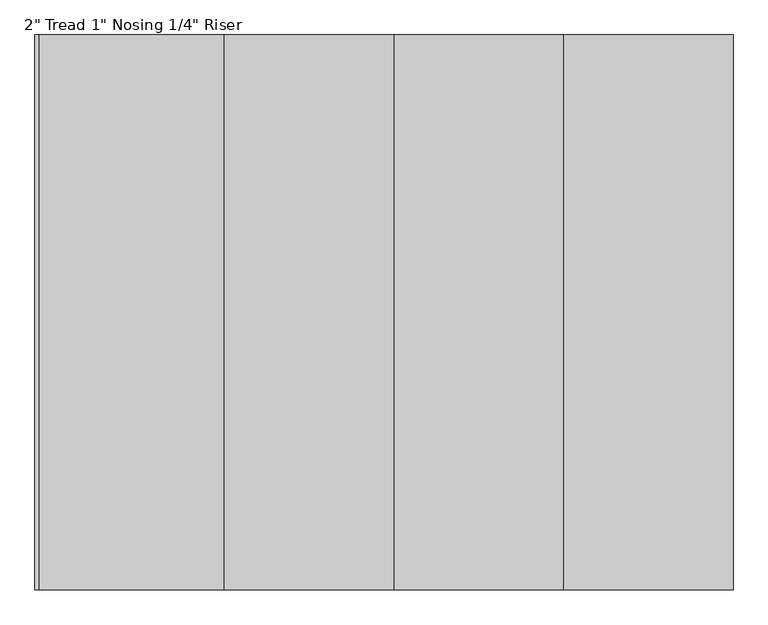
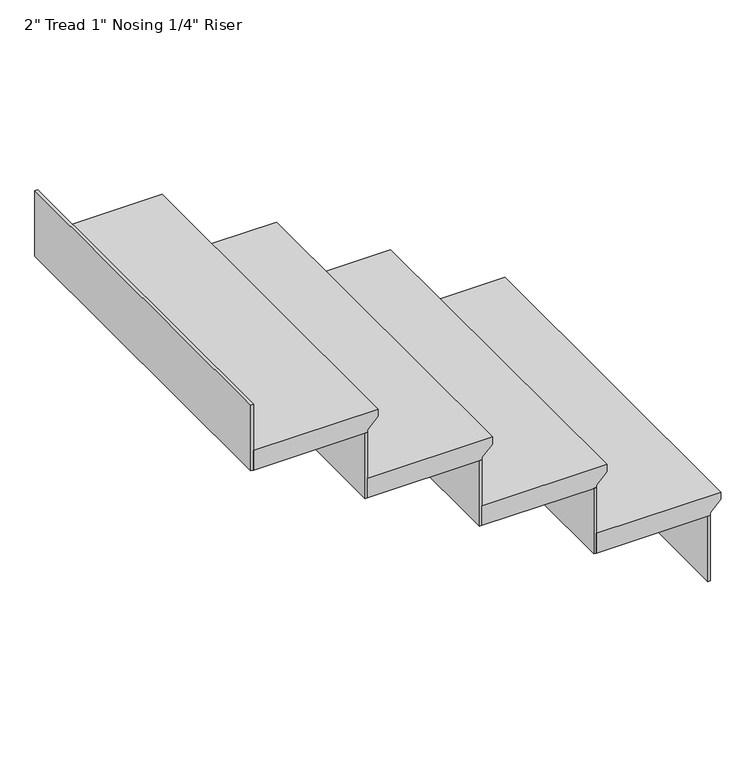
"""IFC4 building model written with IfcOpenShell, lengths in millimetres: stair flight geometry."""

from ifc_helpers import new_model, si_unit, frame, origin, place, context, project, spatial, polyline, outline, extrude, source, transform, mapped, element, save


def stair_flight_6800fc22(model_context):
    return source(origin(), model_context, "Body", "SweptSolid", [
        extrude(outline(polyline([(1016.0, -7602.2399968), (1016.0, -7907.0399968), (965.2, -7907.0399968), (965.2, -7627.6399968), (971.55, -7627.6399968), (996.95, -7602.2399968), (1016.0, -7602.2399968)])), frame((0.0, 8083.4426639, 0.0), z_axis=(0.0, 1.0, 0.0), x_axis=(0.0, 0.0, 1.0)), (0.0, 0.0, 1.0), 914.4),
        extrude(outline(polyline([(-7633.9899968, 8997.8426639), (-7627.6399968, 8997.8426639), (-7627.6399968, 8083.4426639), (-7633.9899968, 8083.4426639), (-7633.9899968, 8997.8426639)])), frame((0.0, 0.0, 795.8666667), z_axis=(0.0, 0.0, 1.0), x_axis=(1.0, 0.0, 0.0)), (0.0, 0.0, 1.0), 169.3333333),
        extrude(outline(polyline([(-7913.3899968, 8997.8426639), (-7907.0399968, 8997.8426639), (-7907.0399968, 8083.4426639), (-7913.3899968, 8083.4426639), (-7913.3899968, 8997.8426639)])), frame((0.0, 0.0, 965.2), z_axis=(0.0, 0.0, 1.0), x_axis=(1.0, 0.0, 0.0)), (0.0, 0.0, 1.0), 169.3333333),
        extrude(outline(polyline([(1185.3333333, -7881.6399968), (1185.3333333, -8186.4399968), (1134.5333333, -8186.4399968), (1134.5333333, -7907.0399968), (1140.8833333, -7907.0399968), (1166.2833333, -7881.6399968), (1185.3333333, -7881.6399968)])), frame((0.0, 8083.4426639, 0.0), z_axis=(0.0, 1.0, 0.0), x_axis=(0.0, 0.0, 1.0)), (0.0, 0.0, 1.0), 914.4),
        extrude(outline(polyline([(-8192.7899968, 8997.8426639), (-8186.4399968, 8997.8426639), (-8186.4399968, 8083.4426639), (-8192.7899968, 8083.4426639), (-8192.7899968, 8997.8426639)])), frame((0.0, 0.0, 1134.5333333), z_axis=(0.0, 0.0, 1.0), x_axis=(1.0, 0.0, 0.0)), (0.0, 0.0, 1.0), 169.3333333),
        extrude(outline(polyline([(1354.6666667, -8161.0399968), (1354.6666667, -8465.8399968), (1303.8666667, -8465.8399968), (1303.8666667, -8186.4399968), (1310.2166667, -8186.4399968), (1335.6166667, -8161.0399968), (1354.6666667, -8161.0399968)])), frame((0.0, 8083.4426639, 0.0), z_axis=(0.0, 1.0, 0.0), x_axis=(0.0, 0.0, 1.0)), (0.0, 0.0, 1.0), 914.4),
        extrude(outline(polyline([(-8472.1899968, 8997.8426639), (-8465.8399968, 8997.8426639), (-8465.8399968, 8083.4426639), (-8472.1899968, 8083.4426639), (-8472.1899968, 8997.8426639)])), frame((0.0, 0.0, 1303.8666667), z_axis=(0.0, 0.0, 1.0), x_axis=(1.0, 0.0, 0.0)), (0.0, 0.0, 1.0), 169.3333333),
        extrude(outline(polyline([(-8751.5899968, 8997.8426639), (-8745.2399968, 8997.8426639), (-8745.2399968, 8083.4426639), (-8751.5899968, 8083.4426639), (-8751.5899968, 8997.8426639)])), frame((0.0, 0.0, 1473.2), z_axis=(0.0, 0.0, 1.0), x_axis=(1.0, 0.0, 0.0)), (0.0, 0.0, 1.0), 169.3333333),
        extrude(outline(polyline([(1524.0, -8440.4399968), (1524.0, -8745.2399968), (1473.2, -8745.2399968), (1473.2, -8465.8399968), (1479.55, -8465.8399968), (1504.95, -8440.4399968), (1524.0, -8440.4399968)])), frame((0.0, 8083.4426639, 0.0), z_axis=(0.0, 1.0, 0.0), x_axis=(0.0, 0.0, 1.0)), (0.0, 0.0, 1.0), 914.4),
    ])


if __name__ == "__main__":
    model = new_model("IFC4")
    model_context = context("Model", 3, world=origin())
    ifc_project = project(units=[si_unit("LENGTHUNIT", "METRE", prefix="MILLI")], contexts=[model_context])
    site = spatial("IfcSite", under=ifc_project)
    building = spatial("IfcBuilding", under=site)
    placement = place(None, origin())
    stair_flight_shape = stair_flight_6800fc22(model_context)
    element("IfcStairFlight", 1, ObjectType="2\" Tread 1\" Nosing 1/4\" Riser", at=placement, inside=building, context=model_context, shape_type="MappedRepresentation", body=[
        mapped(stair_flight_shape, transform((0.0, 0.0, 0.0), x_axis=(1.0, 0.0, 0.0), y_axis=(0.0, 1.0, 0.0), z_axis=(0.0, 0.0, 1.0))),
    ])
    save(model, "model.ifc")
